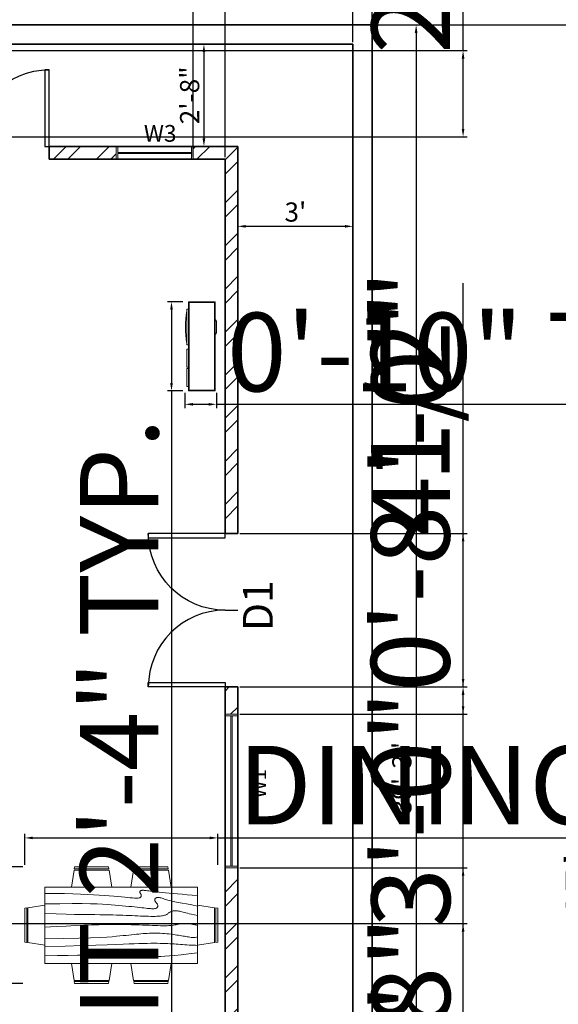
# Model space of a CAD drawing. Units: inches. Extents: x 1542 to 2523, y 1699 to 2449.
# Tile 5 of 7: x 2130 to 2299, y 1984 to 2292. Entities that reach past the tile are written whole.
import ezdxf

# ---------------------------------------------------------------- set-up
doc = ezdxf.new("R2010")
doc.units = ezdxf.units.IN
for name, color, linetype, lineweight in [('A-ANNO-DIMS', 7, 'Continuous', 18), ('A-ANNO-TEXT', 1, 'Continuous', 18), ('A-WALL-PATT', 9, 'Continuous', 13), ('doors', 5, 'Continuous', 25), ('furniture', 9, 'Continuous', 18), ('walls', 7, 'Continuous', 35), ('windows', 93, 'Continuous', 18)]:
    doc.layers.add(name, color=color, linetype=linetype, lineweight=lineweight)
doc.styles.get("Standard").update_dxf_attribs({"font": 'arial.ttf'})
doc.dimstyles.new('ISO-25', dxfattribs={"dimtxt": 24.5625, "dimasz": 2.5, "dimexe": 1.25, "dimexo": 0.625, "dimtad": 1, "dimlunit": 4, "dimtxsty": 'Standard', "dimcen": 2.5, "dimadec": 0, "dimazin": 0, "dimtfac": 10, "dimtmove": 0, "dimatfit": 3, "dimfxl": 1, "dimarcsym": 0})

# ---------------------------------------------------------------- blocks, each defined once
blk = doc.blocks.new('*U2')
for p, q in [((0, 0), (0, -5)), ((30, 0), (30, -5))]:
    blk.add_line(p, q)
blk.add_lwpolyline([(0, 0), (0, 30), (1.75, 30), (1.75, 0)], close=True)
blk.add_arc((0, 0), 30, 0, 90)
blk = doc.blocks.new('Dining Set - 36 x 72 in.')
for p, q in [((-22.2343, 26.00059), (-23.4847, 17.99762)), ((-22.2304, 26), (-5.7608, 26)), ((-22, 27.5), (-22.1562, 26.50042)), ((-5.8416, 26.5), (-22.1534, 26.5)), ((-22, 27.5), (-6, 27.5)), ((-5.8437, 26.49966), (-6, 27.5)), ((-4.5152, 17.99762), (-5.7655, 25.99926)), ((5.7657, 26.00059), (4.5153, 17.99762)), ((5.7696, 26), (22.2392, 26)), ((6, 27.5), (5.8438, 26.50042)), ((22.1584, 26.5), (5.8466, 26.5)), ((6, 27.5), (22, 27.5)), ((22.1563, 26.49966), (22, 27.5)), ((23.4848, 17.99762), (22.2345, 25.99926)), ((36, 18), (-36, 18)), ((-36, 18), (-36, -18)), ((36, -18), (36, 18)), ((-44.0006, 8.23428), (-35.9976, 9.48474)), ((44.0006, 8.23428), (35.9976, 9.48474)), ((-45.5, 8), (-44.5004, 8.15617)), ((-45.5, 8), (-45.5, -8)), ((-44.5, -8.15843), (-44.5, 8.15338)), ((-44, 8.23041), (-44, -8.23915)), ((44, 8.23041), (44, -8.23915)), ((44.5, -8.15843), (44.5, 8.15338)), ((45.5, 8), (44.5005, 8.15617)), ((45.5, 8), (45.5, -8)), ((-44.4997, -8.15631), (-45.5, -8)), ((-35.9976, -9.48476), (-43.9993, -8.2345)), ((35.9976, -9.48476), (43.9993, -8.2345)), ((44.4997, -8.15631), (45.5, -8)), ((-36, -18), (36, -18)), ((-22.2343, -26.0006), (-23.4847, -17.99762)), ((-4.5152, -17.99762), (-5.7655, -25.99928)), ((5.7657, -26.0006), (4.5153, -17.99762)), ((23.4848, -17.99762), (22.2345, -25.99928)), ((-22.2304, -26), (-5.7608, -26)), ((-22, -27.5), (-22.1562, -26.50044)), ((-5.8416, -26.5), (-22.1534, -26.5)), ((-22, -27.5), (-6, -27.5)), ((-5.8437, -26.49967), (-6, -27.5)), ((5.7696, -26), (22.2392, -26)), ((6, -27.5), (5.8438, -26.50044)), ((22.1584, -26.5), (5.8466, -26.5)), ((6, -27.5), (22, -27.5)), ((22.1563, -26.49967), (22, -27.5))]:
    blk.add_line(p, q)
for points in [[(-36, 15), (-31.1772, 14.97754), (-26.8079, 14.91406), (-22.8538, 14.81543), (-19.276, 14.6875), (-16.0362, 14.53613), (-13.0957, 14.36718), (-10.4159, 14.18652), (-7.9583, 14), (-5.6904, 13.81315), (-3.6035, 13.63021), (-1.6954, 13.45508), (0.0365, 13.29166), (1.5945, 13.14388), (2.9811, 13.01562), (4.1988, 12.9108), (5.25, 12.83333), (6.1393, 12.78613), (6.8802, 12.76823), (7.4883, 12.77767), (7.9792, 12.8125), (8.3685, 12.87077), (8.6719, 12.95052), (8.9049, 13.0498), (9.0833, 13.16666), (9.2205, 13.29899), (9.3216, 13.44401), (9.3895, 13.59879), (9.4271, 13.76041), (9.4373, 13.92594), (9.4232, 14.09245), (9.3875, 14.257), (9.3333, 14.41666), (9.2638, 14.56917), (9.1836, 14.71484), (9.0975, 14.85465), (9.0104, 14.98958), (8.9272, 15.1206), (8.8529, 15.2487), (8.7922, 15.37483), (8.75, 15.5), (8.7305, 15.62467), (8.7344, 15.74739), (8.7617, 15.86621), (8.8125, 15.97916), (8.8867, 16.08431), (8.9844, 16.17968), (9.1055, 16.26334), (9.25, 16.33333), (9.4189, 16.38802), (9.6172, 16.42708), (9.8506, 16.45052), (10.125, 16.45833), (10.4463, 16.45052), (10.8203, 16.42708), (11.2529, 16.38802), (11.75, 16.33333), (12.3184, 16.26318), (12.9694, 16.17838), (13.7151, 16.07991), (14.5677, 15.96875), (15.5395, 15.84586), (16.6426, 15.71224), (17.8893, 15.56884), (19.2917, 15.41666), (20.859, 15.25667), (22.5879, 15.08984), (24.4721, 14.91715), (26.5052, 14.73958), (28.6809, 14.5581), (30.9929, 14.3737), (33.4347, 14.18733), (36, 14)], [(-36, 10), (-28.9766, 10.14274), (-23.1725, 10.20442), (-18.4241, 10.19775), (-14.5677, 10.13541), (-11.4399, 10.03011), (-8.877, 9.89453), (-6.7154, 9.74137), (-4.7917, 9.58333), (-2.9698, 9.43082), (-1.2246, 9.28515), (0.4415, 9.14534), (2.026, 9.01041), (3.5266, 8.87939), (4.9408, 8.7513), (6.266, 8.62516), (7.5, 8.5), (8.6411, 8.37549), (9.6914, 8.2539), (10.6538, 8.13818), (11.5312, 8.03125), (12.3267, 7.93603), (13.043, 7.85547), (13.6831, 7.79248), (14.25, 7.75), (14.7471, 7.7303), (15.1797, 7.73307), (15.5537, 7.75732), (15.875, 7.80208), (16.1494, 7.86637), (16.3828, 7.94922), (16.5811, 8.04964), (16.75, 8.16666), (16.8944, 8.29915), (17.0143, 8.44531), (17.1089, 8.60319), (17.1771, 8.77083), (17.218, 8.94629), (17.2305, 9.1276), (17.2137, 9.31282), (17.1667, 9.5), (17.0895, 9.6875), (16.987, 9.875), (16.8649, 10.0625), (16.7292, 10.25), (16.5856, 10.4375), (16.4401, 10.625), (16.2985, 10.8125), (16.1667, 11), (16.05, 11.18733), (15.9518, 11.3737), (15.8752, 11.5581), (15.8229, 11.73958), (15.798, 11.91715), (15.8034, 12.08984), (15.842, 12.25667), (15.9167, 12.41666), (16.0295, 12.56836), (16.1784, 12.70833), (16.3605, 12.83268), (16.5729, 12.9375), (16.8127, 13.01888), (17.0768, 13.07291), (17.3625, 13.0957), (17.6667, 13.08333), (17.9894, 13.03312), (18.3418, 12.94726), (18.7382, 12.82918), (19.1927, 12.68229), (19.7195, 12.51001), (20.3327, 12.31575), (21.0465, 12.10294), (21.875, 11.875), (22.8357, 11.63354), (23.959, 11.37304), (25.2786, 11.08618), (26.8282, 10.76562), (28.6414, 10.40405), (30.752, 9.99414), (33.1936, 9.52856), (36, 9)], [(-36, 5.5), (-30.7157, 5.3348), (-26.069, 5.20963), (-21.9946, 5.11767), (-18.4271, 5.05208), (-15.3009, 5.00602), (-12.5508, 4.97265), (-10.1112, 4.94515), (-7.9167, 4.91666), (-5.909, 4.88167), (-4.0586, 4.83984), (-2.3429, 4.79215), (-0.7396, 4.73958), (0.7739, 4.6831), (2.22, 4.6237), (3.6213, 4.56233), (5, 4.5), (6.373, 4.43782), (7.7344, 4.3776), (9.0723, 4.32129), (10.375, 4.27083), (11.6309, 4.22819), (12.8281, 4.19531), (13.9551, 4.17415), (15, 4.16666), (15.954, 4.17448), (16.819, 4.19791), (17.6001, 4.23698), (18.3021, 4.29166), (18.9299, 4.36198), (19.4883, 4.44791), (19.9823, 4.54948), (20.4167, 4.66666), (20.7969, 4.79899), (21.1302, 4.94401), (21.4245, 5.09879), (21.6875, 5.26041), (21.9271, 5.42594), (22.1511, 5.59245), (22.3672, 5.757), (22.5834, 5.91666), (22.8065, 6.06868), (23.0404, 6.21093), (23.2879, 6.34147), (23.5521, 6.45833), (23.8358, 6.55957), (24.142, 6.64323), (24.4735, 6.70735), (24.8334, 6.75), (25.2235, 6.76969), (25.642, 6.76692), (26.0858, 6.74267), (26.5521, 6.69791), (27.0379, 6.63362), (27.5404, 6.55078), (28.0565, 6.45036), (28.5834, 6.33333), (29.1242, 6.19987), (29.7071, 6.04687), (30.3661, 5.87044), (31.1354, 5.66666), (32.0493, 5.43164), (33.142, 5.16146), (34.4475, 4.85221), (36, 4.5)], [(-36, -1), (-30.7915, -0.6591), (-26.0195, -0.38216), (-21.6519, -0.16284), (-17.6563, 0.00521), (-14.0005, 0.12833), (-10.6523, 0.21289), (-7.5796, 0.26522), (-4.75, 0.29166), (-2.134, 0.29793), (0.2878, 0.28711), (2.5317, 0.26163), (4.6146, 0.22396), (6.5529, 0.17651), (8.3633, 0.12174), (10.0623, 0.06209), (11.6667, 0), (13.1899, -0.06201), (14.6341, -0.1211), (15.9982, -0.17432), (17.2813, -0.21875), (18.4823, -0.25147), (19.6003, -0.26953), (20.6343, -0.27002), (21.5834, -0.25), (22.4481, -0.20768), (23.2357, -0.14584), (23.9549, -0.06836), (24.6146, 0.02083), (25.2235, 0.11784), (25.7904, 0.21875), (26.3241, 0.31966), (26.8334, 0.41666), (27.3265, 0.50618), (27.8099, 0.58593), (28.2894, 0.65397), (28.7709, 0.70833), (29.2601, 0.74707), (29.763, 0.76823), (30.2855, 0.76985), (30.8334, 0.75), (31.4088, 0.70784), (31.9994, 0.64713), (32.589, 0.57275), (33.1615, 0.48958), (33.7008, 0.4025), (34.1908, 0.3164), (34.6153, 0.23616), (34.9584, 0.16666), (35.2099, 0.11165), (35.3848, 0.07031), (35.504, 0.04069), (35.5886, 0.02083), (35.6594, 0.00879), (35.7377, 0.0026), (35.8442, 0.00032), (36, 0)], [(-36, -6.5), (-27.1843, -6.31267), (-20.084, -6.1263), (-14.469, -5.9419), (-10.1094, -5.76042), (-6.7752, -5.58285), (-4.2363, -5.41016), (-2.2629, -5.24333), (-0.625, -5.08334), (0.8708, -4.93099), (2.2715, -4.78646), (3.5872, -4.64974), (4.8281, -4.52084), (6.0046, -4.39974), (7.127, -4.28646), (8.2053, -4.18099), (9.25, -4.08334), (10.2705, -3.99382), (11.2734, -3.91407), (12.2647, -3.84603), (13.25, -3.79167), (14.2354, -3.75293), (15.2266, -3.73177), (16.2295, -3.73015), (17.25, -3.75), (18.2912, -3.79248), (19.3451, -3.85547), (20.4009, -3.93604), (21.4479, -4.03125), (22.4754, -4.13819), (23.4727, -4.25391), (24.4289, -4.37549), (25.3334, -4.5), (26.1785, -4.62492), (26.9694, -4.74935), (27.7145, -4.87281), (28.4219, -4.99479), (29.1, -5.11483), (29.7572, -5.23242), (30.4016, -5.34709), (31.0417, -5.45834), (31.6837, -5.56437), (32.3262, -5.65821), (32.9658, -5.73153), (33.599, -5.77604), (34.2224, -5.78345), (34.8327, -5.74545), (35.4264, -5.65373), (36, -5.5)], [(-36, -10), (-26.4022, -9.81299), (-18.4675, -9.62891), (-11.9839, -9.45069), (-6.7396, -9.28125), (-2.5226, -9.12354), (0.8789, -8.98047), (3.6769, -8.85498), (6.0833, -8.75), (8.2767, -8.66765), (10.3021, -8.60677), (12.1712, -8.56543), (13.8958, -8.54167), (15.4876, -8.53353), (16.9583, -8.53907), (18.3197, -8.55632), (19.5834, -8.58334), (20.7616, -8.61841), (21.8685, -8.66081), (22.9188, -8.71004), (23.9271, -8.76563), (24.9081, -8.82707), (25.8763, -8.89388), (26.8465, -8.96558), (27.8334, -9.04167), (28.8474, -9.12118), (29.8828, -9.20117), (30.93, -9.27824), (31.9792, -9.34896), (33.0205, -9.40991), (34.0443, -9.45768), (35.0407, -9.48885), (36, -9.5)], [(-36, -14.5), (-30.0881, -14.33513), (-25.0332, -14.21224), (-20.7312, -14.12647), (-17.0781, -14.07292), (-13.97, -14.04671), (-11.3027, -14.04297), (-8.9724, -14.05681), (-6.875, -14.08334), (-4.9224, -14.11833), (-3.0905, -14.16016), (-1.3709, -14.20785), (0.2448, -14.26042), (1.7647, -14.3169), (3.1973, -14.3763), (4.5507, -14.43767), (5.8333, -14.5), (7.0554, -14.5621), (8.235, -14.62175), (9.3922, -14.67652), (10.5469, -14.72396), (11.7192, -14.76164), (12.929, -14.78711), (14.1965, -14.79794), (15.5417, -14.79167), (16.9933, -14.76424), (18.6152, -14.70508), (20.4804, -14.60197), (22.6615, -14.44271), (25.2312, -14.21509), (28.2624, -13.9069), (31.8277, -13.50594), (36, -13)]]:
    blk.add_lwpolyline(points)
blk = doc.blocks.new('Entertainment Center')
for p, q in [((-4, 0), (-5, -1)), ((4, 0), (-4, 0)), ((5, -1), (4, 0)), ((-17, -19), (-17, -1)), ((-17, -1), (43, -1)), ((-16.5, -18.5), (-16.5, -1.5)), ((-16.5, -1.5), (42.5, -1.5)), ((42.5, -1.5), (42.5, -18.5)), ((43, -1), (43, -19)), ((43, -19), (-17, -19)), ((42.5, -18.5), (-16.5, -18.5)), ((-12, -20), (-12, -19)), ((12, -19), (12, -20)), ((15, -20), (15, -19)), ((27, -19), (27, -20)), ((28, -20), (28, -19)), ((40, -19), (40, -20)), ((12, -20), (-12, -20)), ((27, -20), (15, -20)), ((40, -20), (28, -20))]:
    blk.add_line(p, q)
blk.add_arc((0, 40), 61, 259.6111, 280.3889)
blk = doc.blocks.new('*D9')
at = {"layer": 'A-ANNO-DIMS', "color": 0, "lineweight": -2, "transparency": 16777216}
for p, q in [((1880.38, 2291.06), (1880.38, 2302.87)), ((1882.88, 2301.62), (2237.88, 2301.62)), ((2240.38, 2291.06), (2240.38, 2302.87))]:
    blk.add_line(p, q, dxfattribs=at)
at = {"layer": 'A-ANNO-DIMS', "color": 0, "transparency": 16777216}
for points in [[(1882.88, 2302.04), (1882.88, 2301.2), (1880.38, 2301.62)], [(2237.88, 2302.04), (2237.88, 2301.2), (2240.38, 2301.62)]]:
    blk.add_solid(points, dxfattribs=at)
at = {"layer": 'Defpoints', "color": 0, "transparency": 16777216}
for p in [(2240.38, 2301.62), (1880.38, 2290.44), (2240.38, 2290.44)]:
    blk.add_point(p, dxfattribs=at)
at = {"layer": 'A-ANNO-DIMS', "color": 0, "transparency": 16777216, "insert": (2060.38, 2308.37), "char_height": 12, "attachment_point": 5}
blk.add_mtext("30'", dxfattribs=at)
blk = doc.blocks.new('*D10')
at = {"layer": 'A-ANNO-DIMS', "color": 0, "lineweight": -2, "transparency": 16777216}
for p, q in [((2241.01, 2290.44), (2316.46, 2290.44)), ((2315.21, 2287.94), (2315.21, 1752.94)), ((2241.01, 1750.44), (2316.46, 1750.44))]:
    blk.add_line(p, q, dxfattribs=at)
at = {"layer": 'A-ANNO-DIMS', "color": 0, "transparency": 16777216}
for points in [[(2314.79, 2287.94), (2315.62, 2287.94), (2315.21, 2290.44)], [(2314.79, 1752.94), (2315.62, 1752.94), (2315.21, 1750.44)]]:
    blk.add_solid(points, dxfattribs=at)
at = {"layer": 'Defpoints', "color": 0, "transparency": 16777216}
for p in [(2240.38, 2290.44), (2240.38, 1750.44), (2315.21, 1750.44)]:
    blk.add_point(p, dxfattribs=at)
at = {"layer": 'A-ANNO-DIMS', "color": 0, "transparency": 16777216, "insert": (2308.48, 2020.44), "char_height": 12, "attachment_point": 5, "rotation": 90}
blk.add_mtext("45'", dxfattribs=at)
blk = doc.blocks.new('*D11')
at = {"layer": 'A-ANNO-DIMS', "color": 0, "lineweight": -2, "transparency": 16777216}
for p, q in [((2241.01, 2290.44), (2255.4, 2290.44)), ((2254.15, 2287.94), (2254.15, 1821.94)), ((2241.01, 1819.44), (2255.4, 1819.44))]:
    blk.add_line(p, q, dxfattribs=at)
at = {"layer": 'A-ANNO-DIMS', "color": 0, "transparency": 16777216}
for points in [[(2253.73, 2287.94), (2254.57, 2287.94), (2254.15, 2290.44)], [(2253.73, 1821.94), (2254.57, 1821.94), (2254.15, 1819.44)]]:
    blk.add_solid(points, dxfattribs=at)
at = {"layer": 'Defpoints', "color": 0, "transparency": 16777216}
for p in [(2240.38, 2290.44), (2240.38, 1819.44), (2254.15, 1819.44)]:
    blk.add_point(p, dxfattribs=at)
at = {"layer": 'A-ANNO-DIMS', "color": 0, "transparency": 16777216, "insert": (2250.46, 2054.94), "char_height": 6, "attachment_point": 5, "rotation": 90}
blk.add_mtext('39\'-3"', dxfattribs=at)
blk = doc.blocks.new('*D12')
at = {"layer": 'A-ANNO-DIMS', "color": 0, "lineweight": -2, "transparency": 16777216}
for p, q in [((2187.19, 2284.44), (2189.02, 2284.44)), ((2187.77, 2281.94), (2187.77, 2254.94)), ((2187.68, 2252.44), (2186.52, 2252.44))]:
    blk.add_line(p, q, dxfattribs=at)
at = {"layer": 'A-ANNO-DIMS', "color": 0, "transparency": 16777216}
for points in [[(2187.35, 2281.94), (2188.19, 2281.94), (2187.77, 2284.44)], [(2187.35, 2254.94), (2188.19, 2254.94), (2187.77, 2252.44)]]:
    blk.add_solid(points, dxfattribs=at)
at = {"layer": 'Defpoints', "color": 0, "transparency": 16777216}
for p in [(2186.56, 2284.44), (2187.77, 2252.44), (2188.31, 2252.44)]:
    blk.add_point(p, dxfattribs=at)
at = {"layer": 'A-ANNO-DIMS', "color": 0, "transparency": 16777216, "insert": (2184.08, 2268.44), "char_height": 6, "attachment_point": 5, "rotation": 90}
blk.add_mtext('2\'-8"', dxfattribs=at)
blk = doc.blocks.new('*D13')
at = {"layer": 'A-ANNO-DIMS', "color": 0, "lineweight": -2, "transparency": 16777216}
for p, q in [((2198.38, 2241.06), (2198.38, 2226.22)), ((2234.38, 2241.06), (2234.38, 2226.22)), ((2200.88, 2227.47), (2231.88, 2227.47))]:
    blk.add_line(p, q, dxfattribs=at)
at = {"layer": 'A-ANNO-DIMS', "color": 0, "transparency": 16777216}
for points in [[(2200.88, 2227.89), (2200.88, 2227.05), (2198.38, 2227.47)], [(2231.88, 2227.89), (2231.88, 2227.05), (2234.38, 2227.47)]]:
    blk.add_solid(points, dxfattribs=at)
at = {"layer": 'Defpoints', "color": 0, "transparency": 16777216}
for p in [(2198.38, 2241.68), (2234.38, 2241.68), (2234.38, 2227.47)]:
    blk.add_point(p, dxfattribs=at)
at = {"layer": 'A-ANNO-DIMS', "color": 0, "transparency": 16777216, "insert": (2216.38, 2231.16), "char_height": 6, "attachment_point": 5}
blk.add_mtext("3'", dxfattribs=at)
blk = doc.blocks.new('WIN-W3-24IN')
for p, q in [((0, 0), (0, 24.03)), ((0, 24.03), (3.94, 24.03)), ((0, 23.53), (3.94, 23.53)), ((1.77, 0.5), (1.77, 23.53)), ((2.17, 0.5), (2.17, 23.53)), ((3.94, 24.03), (3.94, 0)), ((3.94, 0.5), (0, 0.5)), ((3.94, 0), (0, 0))]:
    blk.add_line(p, q)
blk = doc.blocks.new('WIN-W1-48IN')
for p, q in [((0, 0), (0, 48.03)), ((0, 48.03), (3.94, 48.03)), ((0, 47.53), (3.94, 47.53)), ((1.77, 0.5), (1.77, 47.53)), ((2.17, 0.5), (2.17, 47.53)), ((3.94, 48.03), (3.94, 0)), ((3.94, 0.5), (0, 0.5)), ((3.94, 0), (0, 0))]:
    blk.add_line(p, q)
blk = doc.blocks.new('*D27')
at = {"layer": 'A-ANNO-DIMS', "color": 0, "lineweight": -2, "transparency": 16777216}
for p, q in [((2114.72, 2156.7), (2112.11, 2156.7)), ((2113.36, 2154.2), (2113.36, 2148.3)), ((2114.72, 2145.8), (2112.11, 2145.8)), ((2113.36, 2145.8), (2113.36, 1973.25))]:
    blk.add_line(p, q, dxfattribs=at)
at = {"layer": 'A-ANNO-DIMS', "color": 0, "transparency": 16777216}
for points in [[(2112.94, 2154.2), (2113.78, 2154.2), (2113.36, 2156.7)], [(2112.94, 2148.3), (2113.78, 2148.3), (2113.36, 2145.8)]]:
    blk.add_solid(points, dxfattribs=at)
at = {"layer": 'Defpoints', "color": 0, "transparency": 16777216}
for p in [(2115.34, 2156.7), (2113.36, 2145.8), (2115.34, 2145.8)]:
    blk.add_point(p, dxfattribs=at)
at = {"layer": 'A-ANNO-DIMS', "color": 0, "transparency": 16777216, "insert": (2100.19, 2058.28), "char_height": 24.5625, "attachment_point": 5, "rotation": 90}
blk.add_mtext('0\'-11" TYP.', dxfattribs=at)
blk = doc.blocks.new('*D30')
at = {"layer": 'A-ANNO-DIMS', "color": 0, "lineweight": -2, "transparency": 16777216}
for p, q in [((2181.19, 2203.89), (2176.38, 2203.89)), ((2177.63, 2201.39), (2177.63, 2178.49)), ((2181.19, 2175.99), (2176.38, 2175.99)), ((2177.63, 2175.99), (2177.63, 1878.93))]:
    blk.add_line(p, q, dxfattribs=at)
at = {"layer": 'A-ANNO-DIMS', "color": 0, "transparency": 16777216}
for points in [[(2177.21, 2201.39), (2178.05, 2201.39), (2177.63, 2203.89)], [(2177.21, 2178.49), (2178.05, 2178.49), (2177.63, 2175.99)]]:
    blk.add_solid(points, dxfattribs=at)
at = {"layer": 'Defpoints', "color": 0, "transparency": 16777216}
for p in [(2181.81, 2203.89), (2177.63, 2175.99), (2181.81, 2175.99)]:
    blk.add_point(p, dxfattribs=at)
at = {"layer": 'A-ANNO-DIMS', "color": 0, "transparency": 16777216, "insert": (2164.46, 2026.21), "char_height": 24.5625, "attachment_point": 5, "rotation": 90}
blk.add_mtext('TV UNIT 2\'-4" TYP.', dxfattribs=at)
blk = doc.blocks.new('*D31')
at = {"layer": 'A-ANNO-DIMS', "color": 0, "lineweight": -2, "transparency": 16777216}
for p, q in [((2181.81, 2175.37), (2181.81, 2170.56)), ((2191.73, 2175.37), (2191.73, 2170.56)), ((2184.31, 2171.81), (2189.23, 2171.81)), ((2191.73, 2171.81), (2364.28, 2171.81))]:
    blk.add_line(p, q, dxfattribs=at)
at = {"layer": 'A-ANNO-DIMS', "color": 0, "transparency": 16777216}
for points in [[(2184.31, 2172.23), (2184.31, 2171.39), (2181.81, 2171.81)], [(2189.23, 2172.23), (2189.23, 2171.39), (2191.73, 2171.81)]]:
    blk.add_solid(points, dxfattribs=at)
at = {"layer": 'Defpoints', "color": 0, "transparency": 16777216}
for p in [(2181.81, 2175.99), (2191.73, 2175.99), (2191.73, 2171.81)]:
    blk.add_point(p, dxfattribs=at)
at = {"layer": 'A-ANNO-DIMS', "color": 0, "transparency": 16777216, "insert": (2279.26, 2184.97), "char_height": 24.5625, "attachment_point": 5}
blk.add_mtext('0\'-10" TYP.', dxfattribs=at)
blk = doc.blocks.new('*D42')
at = {"layer": 'A-ANNO-DIMS', "color": 0, "lineweight": -2, "transparency": 16777216}
for p, q in [((2131.75, 2027.78), (2131.75, 2037.46)), ((2134.25, 2036.21), (2189.62, 2036.21)), ((2192.12, 2027.78), (2192.12, 2037.46)), ((2192.12, 2036.21), (2523.07, 2036.21))]:
    blk.add_line(p, q, dxfattribs=at)
at = {"layer": 'A-ANNO-DIMS', "color": 0, "transparency": 16777216}
for points in [[(2134.25, 2036.63), (2134.25, 2035.8), (2131.75, 2036.21)], [(2189.62, 2036.63), (2189.62, 2035.8), (2192.12, 2036.21)]]:
    blk.add_solid(points, dxfattribs=at)
at = {"layer": 'Defpoints', "color": 0, "transparency": 16777216}
for p in [(2192.12, 2036.21), (2131.75, 2027.16), (2192.12, 2027.16)]:
    blk.add_point(p, dxfattribs=at)
at = {"layer": 'A-ANNO-DIMS', "color": 0, "transparency": 16777216, "insert": (2358.84, 2049.54), "char_height": 24.5625, "attachment_point": 5}
blk.add_mtext('DINING SET 5\'-0 1/2"', dxfattribs=at)
blk = doc.blocks.new('*D43')
at = {"layer": 'A-ANNO-DIMS', "color": 0, "lineweight": -2, "transparency": 16777216}
for p, q in [((2122.69, 2027.16), (2122.69, 2153.42)), ((2131.12, 2027.16), (2121.44, 2027.16)), ((2122.69, 1993.17), (2122.69, 2024.66)), ((2131.12, 1990.67), (2121.44, 1990.67))]:
    blk.add_line(p, q, dxfattribs=at)
at = {"layer": 'A-ANNO-DIMS', "color": 0, "transparency": 16777216}
for points in [[(2122.28, 2024.66), (2123.11, 2024.66), (2122.69, 2027.16)], [(2122.28, 1993.17), (2123.11, 1993.17), (2122.69, 1990.67)]]:
    blk.add_solid(points, dxfattribs=at)
at = {"layer": 'Defpoints', "color": 0, "transparency": 16777216}
for p in [(2122.69, 2027.16), (2131.75, 2027.16), (2131.75, 1990.67)]:
    blk.add_point(p, dxfattribs=at)
at = {"layer": 'A-ANNO-DIMS', "color": 0, "transparency": 16777216, "insert": (2109.36, 2091.54), "char_height": 24.562, "attachment_point": 5, "rotation": 90}
blk.add_mtext('3\'-0 1/2"', dxfattribs=at)
blk = doc.blocks.new('*D44')
at = {"layer": 'A-ANNO-DIMS', "color": 0, "lineweight": -2, "transparency": 16777216}
for p, q in [((2105.8, 2206.61), (2105.8, 2435.72)), ((2099.19, 2206.61), (2107.05, 2206.61)), ((2105.8, 2160.85), (2105.8, 2204.11)), ((2099.19, 2158.35), (2107.05, 2158.35))]:
    blk.add_line(p, q, dxfattribs=at)
at = {"layer": 'A-ANNO-DIMS', "color": 0, "transparency": 16777216}
for points in [[(2105.39, 2204.11), (2106.22, 2204.11), (2105.8, 2206.61)], [(2105.39, 2160.85), (2106.22, 2160.85), (2105.8, 2158.35)]]:
    blk.add_solid(points, dxfattribs=at)
at = {"layer": 'Defpoints', "color": 0, "transparency": 16777216}
for p in [(2098.56, 2206.61), (2105.8, 2206.61), (2098.56, 2158.35)]:
    blk.add_point(p, dxfattribs=at)
at = {"layer": 'A-ANNO-DIMS', "color": 0, "transparency": 16777216, "insert": (2092.47, 2322.42), "char_height": 24.5625, "attachment_point": 5, "rotation": 90}
blk.add_mtext('SOFA 4\'-0 1/2"', dxfattribs=at)
blk = doc.blocks.new('*D46')
at = {"layer": 'A-ANNO-DIMS', "color": 0, "lineweight": -2, "transparency": 16777216}
for p, q in [((2268.83, 2131.44), (2268.83, 2201.47)), ((2199.01, 2131.44), (2270.08, 2131.44)), ((2268.83, 2085.94), (2268.83, 2128.94)), ((2199.01, 2083.44), (2270.08, 2083.44))]:
    blk.add_line(p, q, dxfattribs=at)
at = {"layer": 'A-ANNO-DIMS', "color": 0, "transparency": 16777216}
for points in [[(2268.42, 2128.94), (2269.25, 2128.94), (2268.83, 2131.44)], [(2268.42, 2085.94), (2269.25, 2085.94), (2268.83, 2083.44)]]:
    blk.add_solid(points, dxfattribs=at)
at = {"layer": 'Defpoints', "color": 0, "transparency": 16777216}
for p in [(2198.38, 2131.44), (2268.83, 2131.44), (2198.38, 2083.44)]:
    blk.add_point(p, dxfattribs=at)
at = {"layer": 'A-ANNO-DIMS', "color": 0, "transparency": 16777216, "insert": (2255.67, 2167.7), "char_height": 24.562, "attachment_point": 5, "rotation": 90}
blk.add_mtext('4\'-0"', dxfattribs=at)
blk = doc.blocks.new('*D47')
at = {"layer": 'A-ANNO-DIMS', "color": 0, "lineweight": -2, "transparency": 16777216}
for p, q in [((2268.83, 2009.44), (2268.83, 2078.47)), ((2071.01, 2009.44), (2270.08, 2009.44)), ((2268.83, 1975.94), (2268.83, 2006.94)), ((2071.01, 1973.44), (2270.08, 1973.44))]:
    blk.add_line(p, q, dxfattribs=at)
at = {"layer": 'A-ANNO-DIMS', "color": 0, "transparency": 16777216}
for points in [[(2268.42, 2006.94), (2269.25, 2006.94), (2268.83, 2009.44)], [(2268.42, 1975.94), (2269.25, 1975.94), (2268.83, 1973.44)]]:
    blk.add_solid(points, dxfattribs=at)
at = {"layer": 'Defpoints', "color": 0, "transparency": 16777216}
for p in [(2070.38, 2009.44), (2268.83, 2009.44), (2070.38, 1973.44)]:
    blk.add_point(p, dxfattribs=at)
at = {"layer": 'A-ANNO-DIMS', "color": 0, "transparency": 16777216, "insert": (2255.66, 2045.2), "char_height": 24.562, "attachment_point": 5, "rotation": 90}
blk.add_mtext('3\'-0"', dxfattribs=at)
blk = doc.blocks.new('*D49')
at = {"layer": 'A-ANNO-DIMS', "color": 0, "lineweight": -2, "transparency": 16777216}
for p, q in [((1851.93, 1958.44), (1851.93, 2027.9)), ((2157.76, 1958.44), (1850.68, 1958.44)), ((1851.93, 1936.94), (1851.93, 1955.94)), ((2157.76, 1934.44), (1850.68, 1934.44))]:
    blk.add_line(p, q, dxfattribs=at)
at = {"layer": 'A-ANNO-DIMS', "color": 0, "transparency": 16777216}
for points in [[(1851.52, 1955.94), (1852.35, 1955.94), (1851.93, 1958.44)], [(1851.52, 1936.94), (1852.35, 1936.94), (1851.93, 1934.44)]]:
    blk.add_solid(points, dxfattribs=at)
at = {"layer": 'Defpoints', "color": 0, "transparency": 16777216}
for p in [(1851.93, 1958.44), (2158.38, 1958.44), (2158.38, 1934.44)]:
    blk.add_point(p, dxfattribs=at)
at = {"layer": 'A-ANNO-DIMS', "color": 0, "transparency": 16777216, "insert": (1838.77, 1994.42), "char_height": 24.562, "attachment_point": 5, "rotation": 90}
blk.add_mtext('2\'-0"', dxfattribs=at)
blk = doc.blocks.new('*D50')
at = {"layer": 'A-ANNO-DIMS', "color": 0, "lineweight": -2, "transparency": 16777216}
for p, q in [((2268.83, 2282.44), (2268.83, 2351.9)), ((1987.01, 2282.44), (2270.08, 2282.44)), ((2268.83, 2257.94), (2268.83, 2279.94)), ((1987.01, 2255.44), (2270.08, 2255.44))]:
    blk.add_line(p, q, dxfattribs=at)
at = {"layer": 'A-ANNO-DIMS', "color": 0, "transparency": 16777216}
for points in [[(2268.42, 2279.94), (2269.25, 2279.94), (2268.83, 2282.44)], [(2268.42, 2257.94), (2269.25, 2257.94), (2268.83, 2255.44)]]:
    blk.add_solid(points, dxfattribs=at)
at = {"layer": 'Defpoints', "color": 0, "transparency": 16777216}
for p in [(1986.38, 2282.44), (2268.83, 2282.44), (1986.38, 2255.44)]:
    blk.add_point(p, dxfattribs=at)
at = {"layer": 'A-ANNO-DIMS', "color": 0, "transparency": 16777216, "insert": (2255.66, 2318.42), "char_height": 24.562, "attachment_point": 5, "rotation": 90}
blk.add_mtext('2\'-3"', dxfattribs=at)
blk = doc.blocks.new('*D54')
at = {"layer": 'A-ANNO-DIMS', "color": 0, "lineweight": -2, "transparency": 16777216}
for p, q in [((2231.88, 2318.89), (2229.38, 2318.89)), ((2234.38, 2285.06), (2234.38, 2320.14)), ((2234.38, 2318.89), (2240.38, 2318.89)), ((2240.38, 2291.06), (2240.38, 2320.14)), ((2242.88, 2318.89), (2311.93, 2318.89))]:
    blk.add_line(p, q, dxfattribs=at)
at = {"layer": 'A-ANNO-DIMS', "color": 0, "transparency": 16777216}
for points in [[(2231.88, 2319.31), (2231.88, 2318.47), (2234.38, 2318.89)], [(2242.88, 2319.31), (2242.88, 2318.47), (2240.38, 2318.89)]]:
    blk.add_solid(points, dxfattribs=at)
at = {"layer": 'Defpoints', "color": 0, "transparency": 16777216}
for p in [(2240.38, 2318.89), (2240.38, 2290.44), (2234.38, 2284.44)]:
    blk.add_point(p, dxfattribs=at)
at = {"layer": 'A-ANNO-DIMS', "color": 0, "transparency": 16777216, "insert": (2278.65, 2332.05), "char_height": 24.562, "attachment_point": 5}
blk.add_mtext('0\'-6"', dxfattribs=at)
blk = doc.blocks.new('*D58')
at = {"layer": 'A-ANNO-DIMS', "color": 0, "lineweight": -2, "transparency": 16777216}
for p, q in [((2268.83, 1898.59), (2268.83, 1987.71)), ((2199.01, 1898.59), (2270.08, 1898.59)), ((2268.83, 1842.94), (2268.83, 1896.09)), ((2199.01, 1840.44), (2270.08, 1840.44))]:
    blk.add_line(p, q, dxfattribs=at)
at = {"layer": 'A-ANNO-DIMS', "color": 0, "transparency": 16777216}
for points in [[(2268.42, 1896.09), (2269.25, 1896.09), (2268.83, 1898.59)], [(2268.42, 1842.94), (2269.25, 1842.94), (2268.83, 1840.44)]]:
    blk.add_solid(points, dxfattribs=at)
at = {"layer": 'Defpoints', "color": 0, "transparency": 16777216}
for p in [(2198.38, 1898.59), (2268.83, 1898.59), (2198.38, 1840.44)]:
    blk.add_point(p, dxfattribs=at)
at = {"layer": 'A-ANNO-DIMS', "color": 0, "transparency": 16777216, "insert": (2255.67, 1944.4), "char_height": 24.562, "attachment_point": 5, "rotation": 90}
blk.add_mtext('4\'-10"', dxfattribs=at)
blk = doc.blocks.new('*D59')
at = {"layer": 'A-ANNO-DIMS', "color": 0, "lineweight": -2, "transparency": 16777216}
for p, q in [((2199.01, 2026.86), (2270.08, 2026.86)), ((2268.83, 1925.12), (2268.83, 2024.36)), ((2199.01, 1922.62), (2270.08, 1922.62))]:
    blk.add_line(p, q, dxfattribs=at)
at = {"layer": 'A-ANNO-DIMS', "color": 0, "transparency": 16777216}
for points in [[(2268.42, 2024.36), (2269.25, 2024.36), (2268.83, 2026.86)], [(2268.42, 1925.12), (2269.25, 1925.12), (2268.83, 1922.62)]]:
    blk.add_solid(points, dxfattribs=at)
at = {"layer": 'Defpoints', "color": 0, "transparency": 16777216}
for p in [(2198.38, 2026.86), (2268.83, 2026.86), (2198.38, 1922.62)]:
    blk.add_point(p, dxfattribs=at)
at = {"layer": 'A-ANNO-DIMS', "color": 0, "transparency": 16777216, "insert": (2255.67, 1974.74), "char_height": 24.562, "attachment_point": 5, "rotation": 90}
blk.add_mtext('8\'-8"', dxfattribs=at)
blk = doc.blocks.new('*D60')
at = {"layer": 'A-ANNO-DIMS', "color": 0, "lineweight": -2, "transparency": 16777216}
for p, q in [((2268.83, 2083.44), (2268.83, 2209.72)), ((2199.01, 2083.44), (2270.08, 2083.44)), ((2268.83, 2077.39), (2268.83, 2080.94)), ((2199.01, 2074.89), (2270.08, 2074.89))]:
    blk.add_line(p, q, dxfattribs=at)
at = {"layer": 'A-ANNO-DIMS', "color": 0, "transparency": 16777216}
for points in [[(2268.42, 2080.94), (2269.25, 2080.94), (2268.83, 2083.44)], [(2268.42, 2077.39), (2269.25, 2077.39), (2268.83, 2074.89)]]:
    blk.add_solid(points, dxfattribs=at)
at = {"layer": 'Defpoints', "color": 0, "transparency": 16777216}
for p in [(2198.38, 2083.44), (2268.83, 2083.44), (2198.38, 2074.89)]:
    blk.add_point(p, dxfattribs=at)
at = {"layer": 'A-ANNO-DIMS', "color": 0, "transparency": 16777216, "insert": (2255.51, 2147.83), "char_height": 24.562, "attachment_point": 5, "rotation": 90}
blk.add_mtext('0\'-8 1/2"', dxfattribs=at)
blk = doc.blocks.new('*D62')
at = {"layer": 'A-ANNO-DIMS', "color": 0, "lineweight": -2, "transparency": 16777216}
for p, q in [((2074.38, 2249.06), (2074.38, 2320.14)), ((2076.88, 2318.89), (2088.88, 2318.89)), ((2091.38, 2249.06), (2091.38, 2320.14)), ((2091.38, 2318.89), (2158.11, 2318.89))]:
    blk.add_line(p, q, dxfattribs=at)
at = {"layer": 'A-ANNO-DIMS', "color": 0, "transparency": 16777216}
for points in [[(2076.88, 2319.31), (2076.88, 2318.47), (2074.38, 2318.89)], [(2088.88, 2319.31), (2088.88, 2318.47), (2091.38, 2318.89)]]:
    blk.add_solid(points, dxfattribs=at)
at = {"layer": 'Defpoints', "color": 0, "transparency": 16777216}
for p in [(2091.38, 2318.89), (2074.38, 2248.44), (2091.38, 2248.44)]:
    blk.add_point(p, dxfattribs=at)
at = {"layer": 'A-ANNO-DIMS', "color": 0, "transparency": 16777216, "insert": (2126, 2332.05), "char_height": 24.562, "attachment_point": 5}
blk.add_mtext('1\'-5"', dxfattribs=at)
blk = doc.blocks.new('*D63')
at = {"layer": 'A-ANNO-DIMS', "color": 0, "lineweight": -2, "transparency": 16777216}
for p, q in [((2184.39, 2249.06), (2184.39, 2320.14)), ((2186.89, 2318.89), (2191.88, 2318.89)), ((2194.38, 2249.06), (2194.38, 2320.14)), ((2194.38, 2318.89), (2282.51, 2318.89))]:
    blk.add_line(p, q, dxfattribs=at)
at = {"layer": 'A-ANNO-DIMS', "color": 0, "transparency": 16777216}
for points in [[(2186.89, 2319.31), (2186.89, 2318.47), (2184.39, 2318.89)], [(2191.88, 2319.31), (2191.88, 2318.47), (2194.38, 2318.89)]]:
    blk.add_solid(points, dxfattribs=at)
at = {"layer": 'Defpoints', "color": 0, "transparency": 16777216}
for p in [(2194.38, 2318.89), (2184.39, 2248.44), (2194.38, 2248.44)]:
    blk.add_point(p, dxfattribs=at)
at = {"layer": 'A-ANNO-DIMS', "color": 0, "transparency": 16777216, "insert": (2239.7, 2332.05), "char_height": 24.562, "attachment_point": 5}
blk.add_mtext('0\'-10"', dxfattribs=at)

msp = doc.modelspace()

# ---------------------------------------------------------------- hatches: boundary and pattern name
at = {"layer": 'A-WALL-PATT'}
h = msp.add_hatch(dxfattribs=at)
h.set_pattern_fill('ANSI32', color=256)
h.paths.add_polyline_path([(2160.362, 2252.439), (2139.383, 2252.439), (2139.383, 2248.439), (2160.362, 2248.439)])
h = msp.add_hatch(dxfattribs=at)
h.set_pattern_fill('ANSI32', color=256)
h.paths.add_polyline_path([(2198.383, 2252.439), (2184.395, 2252.439), (2184.395, 2248.439), (2194.383, 2248.439), (2194.383, 2131.439), (2198.383, 2131.439)])
h = msp.add_hatch(dxfattribs=at)
h.set_pattern_fill('ANSI32', color=256, style=0)
h.paths.add_polyline_path([(2194.383, 2074.895), (2198.383, 2074.895), (2198.383, 2083.439), (2194.383, 2083.439)])
h = msp.add_hatch(dxfattribs=at)
h.set_pattern_fill('ANSI32', color=256)
h.paths.add_polyline_path([(2198.383, 2026.862), (2194.383, 2026.862), (2194.383, 1922.623), (2198.383, 1922.623)])

# ---------------------------------------------------------------- linework, layer by layer
at = {"layer": 'walls'}
for p, q in [((1880.383, 2290.439), (2240.383, 2290.439)), ((2240.383, 2290.439), (2240.383, 1819.439)), ((1886.383, 2284.439), (2234.383, 2284.439)), ((2234.383, 2284.439), (2234.383, 1819.439)), ((2198.383, 2252.439), (2139.383, 2252.439)), ((2139.383, 2252.439), (2139.383, 2248.439)), ((2198.383, 2252.439), (2198.383, 2131.439)), ((2194.383, 2248.439), (2139.383, 2248.439)), ((2194.383, 2248.439), (2194.383, 2131.439)), ((2198.383, 2131.439), (2194.383, 2131.439)), ((2194.383, 2083.439), (2198.383, 2083.439)), ((2194.383, 2083.439), (2194.383, 1844.439)), ((2198.383, 2083.439), (2194.383, 2083.439)), ((2198.383, 2083.439), (2198.383, 1840.439))]:
    msp.add_line(p, q, dxfattribs=at)

# ---------------------------------------------------------------- block references
at = {"layer": 'doors', "xscale": -0.8, "yscale": 0.8, "zscale": 0.8}
msp.add_blockref('*U2', (2139.383, 2252.439), dxfattribs=at)
at = {"layer": 'doors', "yscale": 0.8, "zscale": 0.8, "rotation": 90}
for p, xscale in [((2194.383, 2131.439), -0.8), ((2194.383, 2083.439), 0.8)]:
    msp.add_blockref('*U2', p, dxfattribs=dict(at, xscale=xscale))
at = {"layer": 'furniture', "xscale": 0.4648726153281338, "yscale": 0.4648726153281338, "zscale": 0.4648726153281338, "rotation": 270}
msp.add_blockref('Entertainment Center', (2191.731, 2195.982), dxfattribs=at)
at = {"layer": 'furniture', "xscale": 0.6633856142375758, "yscale": 0.6633856142375758, "zscale": 0.6633856142375758}
msp.add_blockref('Dining Set - 36 x 72 in.', (2161.934, 2008.917), dxfattribs=at)
at = {"layer": 'windows'}
for name, p, rotation in [('WIN-W3-24IN', (2184.395, 2248.439), 89.99999999999666), ('WIN-W1-48IN', (2198.383, 2074.894), 180)]:
    msp.add_blockref(name, p, dxfattribs=dict(at, rotation=rotation))

# ---------------------------------------------------------------- texts
at = {"layer": 'A-ANNO-TEXT', "insert": (2168.984, 2259.16), "char_height": 5.2329, "attachment_point": 1}
msp.add_mtext_dynamic_manual_height_columns('W3', width=1.62225, gutter_width=26.164, heights=[0], dxfattribs=at)
at = {"layer": 'A-ANNO-TEXT', "attachment_point": 1, "rotation": 90}
for s, width, gutter_width, insert, char_height in [('D1', 3.38383, 46.636, (2199.985, 2100.924), 9.3273), ('W1', 1.45099, 23.402, (2202.532, 2048.561), 4.6805)]:
    msp.add_mtext_dynamic_manual_height_columns(s, width=width, gutter_width=gutter_width, heights=[0], dxfattribs=dict(at, insert=insert, char_height=char_height))

# ---------------------------------------------------------------- dimensions: what is measured, and where the dimension line sits
at = {"layer": 'A-ANNO-DIMS'}
for base, p1, p2, angle, text, picture, middle in [((2105.802, 2206.606), (2098.565, 2158.354), (2098.565, 2206.606), 90, 'SOFA <>', '*D44', (2092.469, 2322.416)), ((2177.629, 2175.993), (2181.813, 2203.885), (2181.813, 2175.993), 270, 'TV UNIT <> TYP.', '*D30', (2164.463, 2026.213)), ((2113.36, 2145.804), (2115.34, 2156.705), (2115.34, 2145.804), 270, '<> TYP.', '*D27', (2100.194, 2058.277))]:
    dim = msp.add_linear_dim(base=base, p1=p1, p2=p2, angle=angle, text=text, dimstyle='ISO-25', override={"dimdec": 1, "dimlfac": 1, "dimrnd": 0, "dimzin": 1, "dimdsep": 46, "dimlunit": 4, "dimfrac": 2}, dxfattribs=at)
    dim.commit()
    dim.dimension.update_dxf_attribs({"geometry": picture, "text_midpoint": middle})
for base, p1, p2, override, picture, middle in [((2268.833, 2282.439), (1986.383, 2255.439), (1986.383, 2282.439), {"dimdec": 1, "dimlfac": 1, "dimrnd": 0, "dimzin": 1, "dimdsep": 46, "dimlunit": 4, "dimfrac": 2}, '*D50', (2255.658, 2318.42)), ((2315.207, 1750.439), (2240.383, 2290.439), (2240.383, 1750.439), {"dimtxt": 12, "dimclrd": 0, "dimclre": 0, "dimclrt": 0}, '*D10', (2308.48, 2020.439)), ((2254.15, 1819.439), (2240.383, 2290.439), (2240.383, 1819.439), {"dimtxt": 6, "dimclrd": 0, "dimclre": 0, "dimclrt": 0}, '*D11', (2250.459, 2054.939)), ((2187.769, 2252.439), (2186.562, 2284.439), (2188.306, 2252.439), {"dimtxt": 6, "dimclrd": 0, "dimclre": 0, "dimclrt": 0}, '*D12', (2184.081, 2268.439)), ((2268.833, 2083.439), (2198.383, 2074.895), (2198.383, 2083.439), {"dimdec": 1, "dimlfac": 1, "dimrnd": 0, "dimzin": 1, "dimdsep": 46, "dimlunit": 4, "dimfrac": 2}, '*D60', (2255.507, 2147.828)), ((2268.833, 2131.439), (2198.383, 2083.439), (2198.383, 2131.439), {"dimdec": 1, "dimlfac": 1, "dimrnd": 0, "dimzin": 1, "dimdsep": 46, "dimlunit": 4, "dimfrac": 2}, '*D46', (2255.667, 2167.705)), ((2122.695, 2027.16), (2131.75, 1990.673), (2131.75, 2027.16), {"dimdec": 1, "dimlfac": 1, "dimrnd": 0, "dimzin": 1, "dimdsep": 46, "dimlunit": 4, "dimfrac": 2}, '*D43', (2109.361, 2091.54)), ((2268.833, 2009.439), (2070.383, 1973.439), (2070.383, 2009.439), {"dimdec": 1, "dimlfac": 1, "dimrnd": 0, "dimzin": 1, "dimdsep": 46, "dimlunit": 4, "dimfrac": 2}, '*D47', (2255.658, 2045.202)), ((1851.933, 1958.439), (2158.383, 1934.439), (2158.383, 1958.439), {"dimdec": 1, "dimlfac": 1, "dimrnd": 0, "dimzin": 1, "dimdsep": 46, "dimlunit": 4, "dimfrac": 2}, '*D49', (1838.767, 1994.42)), ((2268.833, 2026.862), (2198.383, 1922.623), (2198.383, 2026.862), {"dimdec": 1, "dimlfac": 1, "dimrnd": 0, "dimzin": 1, "dimdsep": 46, "dimlunit": 4, "dimfrac": 2}, '*D59', (2255.667, 1974.743)), ((2268.833, 1898.591), (2198.383, 1840.439), (2198.383, 1898.591), {"dimdec": 1, "dimlfac": 1, "dimrnd": 0, "dimzin": 1, "dimdsep": 46, "dimlunit": 4, "dimfrac": 2}, '*D58', (2255.667, 1944.399))]:
    dim = msp.add_linear_dim(base=base, p1=p1, p2=p2, angle=90, dimstyle='ISO-25', override=override, dxfattribs=at)
    dim.commit()
    dim.dimension.update_dxf_attribs({"geometry": picture, "text_midpoint": middle})
for base, p1, p2, override, picture, middle in [((2091.383, 2318.889), (2074.383, 2248.439), (2091.383, 2248.439), {"dimdec": 1, "dimlfac": 1, "dimrnd": 0, "dimzin": 1, "dimdsep": 46, "dimlunit": 4, "dimfrac": 2}, '*D62', (2125.998, 2332.055)), ((2194.383, 2318.889), (2184.395, 2248.439), (2194.383, 2248.439), {"dimdec": 1, "dimlfac": 1, "dimrnd": 0, "dimzin": 1, "dimdsep": 46, "dimlunit": 4, "dimfrac": 2}, '*D63', (2239.696, 2332.055)), ((2240.383, 2318.889), (2234.383, 2284.439), (2240.383, 2290.439), {"dimdec": 1, "dimlfac": 1, "dimrnd": 0, "dimzin": 1, "dimdsep": 46, "dimlunit": 4, "dimfrac": 2}, '*D54', (2278.654, 2332.055)), ((2240.383, 2301.619), (1880.383, 2290.439), (2240.383, 2290.439), {"dimtxt": 12, "dimclrd": 0, "dimclre": 0, "dimclrt": 0}, '*D9', (2060.383, 2308.375)), ((2234.383, 2227.471), (2198.383, 2241.682), (2234.383, 2241.682), {"dimtxt": 6, "dimclrd": 0, "dimclre": 0, "dimclrt": 0}, '*D13', (2216.383, 2231.161))]:
    dim = msp.add_linear_dim(base=base, p1=p1, p2=p2, dimstyle='ISO-25', override=override, dxfattribs=at)
    dim.commit()
    dim.dimension.update_dxf_attribs({"geometry": picture, "text_midpoint": middle})
for base, p1, p2, text, picture, middle in [((2191.731, 2171.809), (2181.813, 2175.993), (2191.731, 2175.993), '<> TYP.', '*D31', (2279.258, 2184.975)), ((2192.118, 2036.215), (2131.75, 2027.16), (2192.118, 2027.16), 'DINING SET <>', '*D42', (2358.845, 2049.54))]:
    dim = msp.add_linear_dim(base=base, p1=p1, p2=p2, text=text, dimstyle='ISO-25', override={"dimdec": 1, "dimlfac": 1, "dimrnd": 0, "dimzin": 1, "dimdsep": 46, "dimlunit": 4, "dimfrac": 2}, dxfattribs=at)
    dim.commit()
    dim.dimension.update_dxf_attribs({"geometry": picture, "text_midpoint": middle})

doc.saveas('drawing.dxf')
